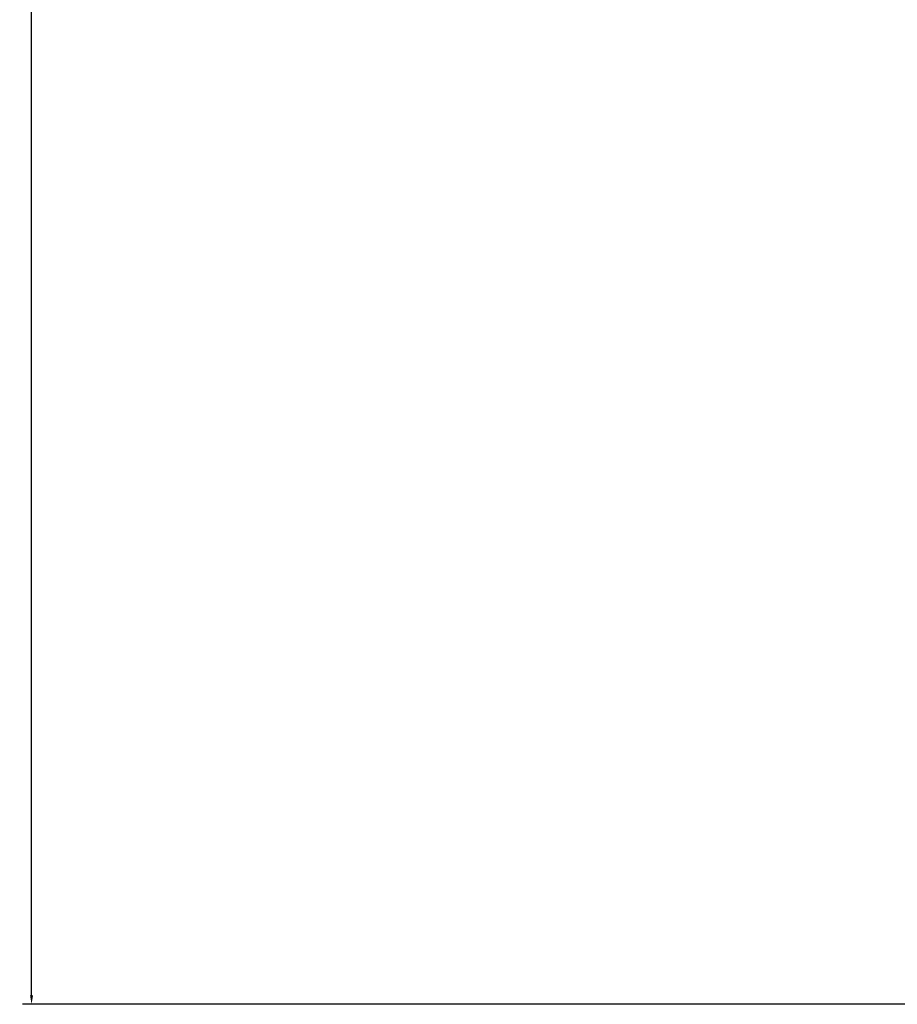
# Model space of a CAD drawing. Units: inches. Extents: x 738 to 1068, y 378 to 757.
# Tile 1 of 41: x 738 to 756, y 396 to 416. Entities that reach past the tile are written whole.
import ezdxf

# ---------------------------------------------------------------- set-up
doc = ezdxf.new("R2010")
doc.units = ezdxf.units.IN
doc.header["$MEASUREMENT"] = 0
doc.layers.add('A-ANNO-DIMS', color=2, linetype='Continuous', lineweight=18)
doc.styles.get("Standard").update_dxf_attribs({"font": 'arial.ttf'})
doc.dimstyles.get("Standard").update_dxf_attribs({"dimtxt": 0.18, "dimasz": 0.18, "dimexe": 0.18, "dimexo": 0.0625, "dimgap": 0.09, "dimtad": 0, "dimtih": 1, "dimtoh": 1, "dimdec": 4, "dimzin": 0, "dimdsep": 46, "dimtxsty": 'Standard', "dimcen": 0.09, "dimadec": 0, "dimazin": 0, "dimtfac": 1, "dimtdec": 4, "dimtofl": 0, "dimtmove": 0, "dimatfit": 3, "dimfxl": 1, "dimtolj": 1, "dimtzin": 0, "dimarcsym": 0})

# ---------------------------------------------------------------- blocks, each defined once
blk = doc.blocks.new('*D19')
at = {"layer": 'A-ANNO-DIMS', "color": 0, "lineweight": -2, "transparency": 16777216}
for p, q in [((781.422, 446.265), (738.194, 446.265)), ((738.374, 446.085), (738.374, 421.499)), ((738.374, 396.549), (738.374, 421.135)), ((781.385, 396.369), (738.194, 396.369))]:
    blk.add_line(p, q, dxfattribs=at)
at = {"layer": 'A-ANNO-DIMS', "color": 0, "transparency": 16777216}
for points in [[(738.344, 446.085), (738.404, 446.085), (738.374, 446.265)], [(738.344, 396.549), (738.404, 396.549), (738.374, 396.369)]]:
    blk.add_solid(points, dxfattribs=at)
at = {"layer": 'Defpoints', "color": 0, "transparency": 16777216}
for p in [(738.374, 446.265), (781.485, 446.265), (781.447, 396.369)]:
    blk.add_point(p, dxfattribs=at)
at = {"layer": 'A-ANNO-DIMS', "color": 0, "transparency": 16777216, "insert": (738.374, 421.317), "char_height": 0.18, "attachment_point": 5}
blk.add_mtext('\\A1;49.9', dxfattribs=at)

msp = doc.modelspace()

# ---------------------------------------------------------------- dimensions: what is measured, and where the dimension line sits
at = {"layer": 'A-ANNO-DIMS'}
dim = msp.add_linear_dim(base=(738.3736, 446.2651), p1=(781.4474, 396.3691), p2=(781.4846, 446.2651), angle=90, dimstyle='Standard', override={"dimdec": 1, "dimlfac": 1, "dimrnd": 0, "dimzin": 0, "dimdsep": 46, "dimlunit": 2}, dxfattribs=at)
dim.commit()
dim.dimension.update_dxf_attribs({"geometry": '*D19', "text_midpoint": (738.3736, 421.3171)})

doc.saveas('drawing.dxf')
